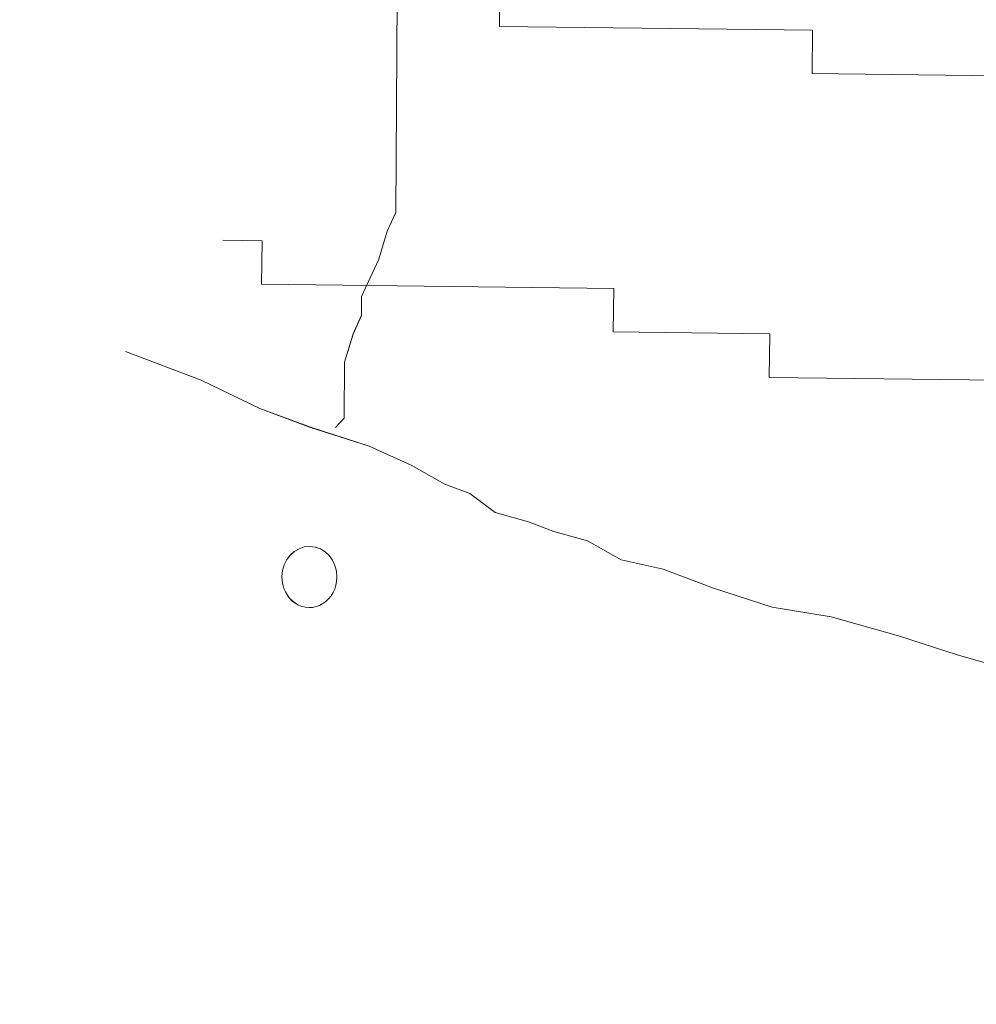
# Model space of a CAD drawing. Units: inches. Extents: x -466983 to 1020, y 324 to 318697.
# Tile 54 of 97: x 631.804 to 634.844, y 939.565 to 942.694. Entities that reach past the tile are written whole.
import ezdxf

# ---------------------------------------------------------------- set-up
doc = ezdxf.new("R2010")
doc.units = ezdxf.units.IN
doc.header["$MEASUREMENT"] = 0
doc.layers.add('A-FLOR-PATT', color=252, linetype='Continuous', lineweight=13)
doc.layers.add('A-FURN', color=8, linetype='Continuous', lineweight=18)

# ---------------------------------------------------------------- blocks, each defined once
blk = doc.blocks.new('L Shaped Sofa')
at = {"ltscale": 2}
for p, q in [((2434.5891, 747.5867), (2435.1737, 747.4213)), ((2435.1737, 747.4213), (2435.5146, 747.3113)), ((2435.5146, 747.3113), (2435.9043, 747.201)), ((2435.9043, 747.201), (2436.2455, 747.1452)), ((2436.2455, 747.1452), (2436.5864, 747.0351)), ((2436.5864, 747.0351), (2436.8785, 746.9253)), ((2436.8785, 746.9253), (2437.1222, 746.87)), ((2437.1222, 746.87), (2437.3167, 746.7606)), ((2437.3167, 746.7606), (2437.5115, 746.7055)), ((2437.5115, 746.7055), (2437.6576, 746.6506)), ((2437.6576, 746.6506), (2437.8524, 746.5955)), ((2437.8524, 746.5955), (2437.9981, 746.4863)), ((2437.9981, 746.4863), (2438.1442, 746.4314)), ((2438.1442, 746.4314), (2438.3387, 746.3221)), ((2438.3387, 746.3221), (2438.582, 746.2125)), ((2438.582, 746.2125), (2438.9229, 746.1025)), ((2438.7274, 746.0492), (2438.7765, 746.1032)), ((2438.9229, 746.1025), (2439.215, 745.9927)), ((2438.7254, 745.7239), (2438.7274, 746.0492)), ((2439.215, 745.9927), (2439.5556, 745.8284)), ((2434.2218, 745.8377), (2436.2633, 745.8128)), ((2436.2633, 745.8128), (2436.2603, 745.5609)), ((2439.5556, 745.8284), (2439.9938, 745.6637)), ((2438.6756, 745.5615), (2438.7254, 745.7239)), ((2436.2603, 745.5609), (2437.1676, 745.5498)), ((2438.6262, 745.4533), (2438.6756, 745.5615)), ((2437.1676, 745.5498), (2437.1645, 745.2979)), ((2438.6255, 745.3448), (2438.6262, 745.4533)), ((2438.5266, 745.1284), (2438.6255, 745.3448)), ((2437.1645, 745.2979), (2439.2061, 745.2729)), ((2439.2061, 745.2729), (2439.203, 745.021)), ((2438.4768, 744.966), (2438.5266, 745.1284)), ((2439.4298, 745.0182), (2439.203, 745.021)), ((2439.203, 745.021), (2439.4298, 745.0182)), ((2438.4273, 744.8578), (2438.4768, 744.966)), ((2438.4141, 742.6892), (2438.4273, 744.8578)), ((2433.5198, 744.0827), (2436.015, 744.0522)), ((2436.015, 744.0522), (2436.0119, 743.8003)), ((2436.0119, 743.8003), (2437.8266, 743.7781)), ((2437.8266, 743.7781), (2437.8235, 743.5262))]:
    blk.add_line(p, q, dxfattribs=at)
at = {"ltscale": 2, "extrusion": (0, 0, -1)}
for start_param, end_param in [(1.570796, 4.712389), (-1.570796, 1.570796)]:
    blk.add_ellipse((2438.9282, 746.9699), major_axis=(-0.0022, -0.1772), ratio=0.9, start_param=start_param, end_param=end_param, dxfattribs=at)

msp = doc.modelspace()

# ---------------------------------------------------------------- hatches: boundary and pattern name
at = {"layer": 'A-FLOR-PATT', "transparency": 33554572}
h = msp.add_hatch(dxfattribs=at)
h.set_pattern_fill('ANSI37', color=256, scale=30)
h.set_pattern_definition([(45, (-1212.4137, -290.035), (-2.6516504, 2.6516504), []), (135, (-1212.4137, -290.035), (-2.6516504, -2.6516504), [])])
h.paths.add_polyline_path([(901.8057, 1075.9377), (900.6144, 1075.9377), (900.6144, 1065.3856), (899.391, 1065.3856), (898.0911, 1065.3856), (892.8356, 1058.7098, -0.258377), (892.1875, 1058.3509), (879.9848, 1058.3509, -0.20177), (879.4382, 1058.5808), (874.0812, 1065.3856), (872.7813, 1065.3856), (871.5579, 1065.3856), (871.5579, 1075.9377), (813.8057, 1075.9377), (813.8057, 1044.7922), (832.3947, 1044.7922, -0.394795), (848.6602, 1028.5356), (848.6602, 1009.9377), (901.8057, 1009.9377), (901.8057, 1015.9377), (901.3057, 1015.9377), (871.3057, 1015.9377), (871.3057, 1017.2502), (871.3344, 1017.2502, -0.401453), (901.3057, 1045.9377), (901.8057, 1045.9377)])
edge = h.paths.add_edge_path(flags=16)
edge.add_line((847.7731, 1068.9486), (847.7731, 1073.7088))
edge.add_arc((849.2269, 1073.7088), 1.4538, 90, 180, ccw=False)
edge.add_line((849.2269, 1075.1627), (864.4921, 1075.1627))
edge.add_arc((864.4921, 1073.7088), 1.4538, 0, 90, ccw=False)
edge.add_line((865.9459, 1073.7088), (865.9459, 1069.0035))
edge.add_arc((832.6447, 1068.9761), 33.3012, -20.61234, 0.04725, ccw=False)
edge.add_ellipse((856.8595, 1058.48), major_axis=(0, 10.2131), ratio=0.6859192, start_angle=100.00884, end_angle=259.99116, ccw=False)
edge.add_arc((881.0742, 1068.9761), 33.3012, 180.04725, 200.61234, ccw=False)
h.paths.add_polyline_path([(853.1456, 1066.4815), (853.1456, 1066.4534), (853.1463, 1066.4534, 0.433107), (852.9166, 1066.6849), (852.9166, 1066.4534), (853.1456, 1066.4534), (853.1456, 1066.4815), (853.088, 1066.6122, 0.697939), (852.6995, 1066.4534), (852.7003, 1066.4534), (852.7003, 1066.4815), (852.9166, 1067.0012), (852.9166, 1066.6849, -0.396254)], flags=0)
h.paths.add_polyline_path([(861.0187, 1066.4815), (861.0187, 1066.4534), (861.0194, 1066.4534, 0.416404), (860.8024, 1066.6849), (860.8024, 1066.4534), (861.0187, 1066.4534), (861.0187, 1066.4815), (860.9672, 1066.6053, 0.713344), (860.5726, 1066.4534), (860.5734, 1066.4534), (860.5734, 1066.4815), (860.8024, 1067.0012), (860.8024, 1066.6849, -0.379973)], flags=0)
edge = h.paths.add_edge_path(flags=0)
edge.add_spline(control_points=[(861.1298, 1065.7855), (861.4661, 1065.2478), (861.6134, 1065.0161), (861.9833, 1064.3736), (862.1924, 1063.9443), (862.5614, 1063.0391), (862.7212, 1062.5633), (862.9865, 1061.5781), (863.092, 1061.0689), (863.2452, 1060.031), (863.293, 1059.5025), (863.3295, 1058.4409), (863.3181, 1057.9078), (863.2366, 1056.8518), (863.1664, 1056.3289), (862.9695, 1055.308), (862.8427, 1054.8099), (862.5365, 1053.8522), (862.3571, 1053.3927), (861.9514, 1052.5249), (861.7251, 1052.1166), (861.233, 1051.3622), (860.9672, 1051.0162), (860.4048, 1050.3949), (860.1082, 1050.1197), (859.4937, 1049.6461), (859.1758, 1049.4476), (858.5276, 1049.1299), (858.1973, 1049.0107), (857.5315, 1048.8518), (857.1959, 1048.8121), (856.5249, 1048.812), (856.1894, 1048.8515), (855.5236, 1049.0101), (855.1933, 1049.1291), (854.545, 1049.4465), (854.2271, 1049.6449), (853.6124, 1050.1183), (853.3158, 1050.3933), (852.7533, 1051.0143), (852.4874, 1051.3602), (851.9952, 1052.1144), (851.7688, 1052.5225), (851.3629, 1053.3902), (851.1834, 1053.8496), (850.877, 1054.8071), (850.7501, 1055.3051), (850.553, 1056.326), (850.4827, 1056.8488), (850.401, 1057.9048), (850.3895, 1058.4379), (850.4257, 1059.4995), (850.4734, 1060.0281), (850.6265, 1061.066), (850.7318, 1061.5753), (850.9969, 1062.5605), (851.1567, 1063.0365), (851.5254, 1063.9418), (851.7345, 1064.3712), (852.1056, 1065.0164), (852.2544, 1065.2503), (852.6082, 1065.7335)], knot_values=[3.915332, 3.915332, 3.915332, 3.915332, 4.013468, 4.013468, 4.175532, 4.175532, 4.337596, 4.337596, 4.49966, 4.49966, 4.661724, 4.661724, 4.823788, 4.823788, 4.985852, 4.985852, 5.147916, 5.147916, 5.30998, 5.30998, 5.472044, 5.472044, 5.634109, 5.634109, 5.796173, 5.796173, 5.958237, 5.958237, 6.120301, 6.120301, 6.282365, 6.282365, 6.444429, 6.444429, 6.606493, 6.606493, 6.768557, 6.768557, 6.930621, 6.930621, 7.092685, 7.092685, 7.254749, 7.254749, 7.416813, 7.416813, 7.578878, 7.578878, 7.740942, 7.740942, 7.903006, 7.903006, 8.06507, 8.06507, 8.227134, 8.227134, 8.389198, 8.389198, 8.551262, 8.551262, 8.65037, 8.65037, 8.65037, 8.65037], degree=3, periodic=0)
edge.add_line((852.6421, 1065.7855), (861.1298, 1065.7855))
edge = h.paths.add_edge_path(flags=0)
edge.add_ellipse((856.8496, 1057.7432), major_axis=(0, 7.7921), ratio=0.687861, start_angle=0, end_angle=360)
h.paths.add_polyline_path([(848.8634, 1069.3891), (848.8634, 1073.9605, -0.414214), (849.9538, 1075.0508), (863.7652, 1075.0508, -0.414214), (864.8555, 1073.9605), (864.8555, 1069.3891, -0.388936), (864.5237, 1069.027, -0.043561), (849.1953, 1069.027, -0.388936)], flags=0)
h.paths.add_polyline_path([(853.1006, 1068.1122, -1), (852.6775, 1068.1122, -1)], flags=0)
edge = h.paths.add_edge_path(flags=0)
edge.add_ellipse((856.8595, 1057.3378), major_axis=(0, 2.207), ratio=0.657164, start_angle=0, end_angle=360)
h.paths.add_polyline_path([(861.0415, 1068.1122, -1), (860.6184, 1068.1122, -1)], flags=0)
edge = h.paths.add_edge_path()
edge.add_line((573.9537, 1057.3412), (573.9537, 1075.9377))
edge.add_line((573.9537, 1075.9377), (558.7308, 1075.9377))
edge.add_line((558.7308, 1075.9377), (558.7308, 1065.3856))
edge.add_line((558.7308, 1065.3856), (557.5074, 1065.3856))
edge.add_line((557.5074, 1065.3856), (556.2075, 1065.3856))
edge.add_line((556.2075, 1065.3856), (550.952, 1058.7098))
edge.add_arc((550.3039, 1059.1155), 0.7646, 270, 327.9483, ccw=False)
edge.add_line((550.3039, 1058.3509), (538.1012, 1058.3509))
edge.add_arc((538.1012, 1059.1155), 0.7646, 224.3704, 270, ccw=False)
edge.add_line((537.5546, 1058.5808), (532.1976, 1065.3856))
edge.add_line((532.1976, 1065.3856), (530.8977, 1065.3856))
edge.add_line((530.8977, 1065.3856), (529.6743, 1065.3856))
edge.add_line((529.6743, 1065.3856), (529.6743, 1075.9377))
edge.add_line((529.6743, 1075.9377), (520.8057, 1075.9377))
edge.add_line((520.8057, 1075.9377), (520.8057, 1045.9377))
edge.add_line((520.8057, 1045.9377), (521.3057, 1045.9377))
edge.add_arc((521.3057, 1015.9377), 30, 2.50749, 90, ccw=False)
edge.add_line((551.277, 1017.2502), (551.3057, 1017.2502))
edge.add_line((551.3057, 1017.2502), (551.3057, 1015.9377))
edge.add_line((551.3057, 1015.9377), (520.8057, 1015.9377))
edge.add_line((520.8057, 1015.9377), (520.8057, 1009.9377))
edge.add_line((520.8057, 1009.9377), (559.1913, 1010.4022))
edge.add_arc((559.1913, 1011.856), 1.4538, 180, 270, ccw=False)
edge.add_line((557.7375, 1011.856), (557.7375, 1016.5613))
edge.add_arc((591.0386, 1016.5888), 33.3012, 159.38766, 180.04725, ccw=False)
edge.add_ellipse((566.8239, 1027.0848), major_axis=(0, 10.2131), ratio=0.6859192, start_angle=280.00884, end_angle=439.99116, ccw=False)
edge.add_arc((542.6091, 1016.5888), 33.3012, 0.04725, 20.61234, ccw=False)
edge.add_line((575.9103, 1016.6162), (575.9103, 1011.856))
edge.add_arc((574.4565, 1011.856), 1.4538, -90, 0, ccw=False)
edge.add_line((574.4565, 1010.4022), (608.8057, 1009.9377))
edge.add_line((608.8057, 1009.9377), (608.8057, 1041.0857))
edge.add_line((608.8057, 1041.0857), (590.2179, 1041.0857))
edge.add_arc((590.775, 1057.9074), 16.8309, 181.92775, 268.10321, ccw=False)
edge = h.paths.add_edge_path()
edge.add_ellipse((494.2443, 583.6204), major_axis=(0, 10.2131), ratio=0.6859192, start_angle=280.00884, end_angle=439.99116, ccw=False)
edge.add_arc((470.0296, 573.1243), 33.3012, 0.04725, 20.61234, ccw=False)
edge.add_line((503.3307, 573.1518), (503.3307, 568.3916))
edge.add_arc((501.8769, 568.3916), 1.4538, -90, 0, ccw=False)
edge.add_line((501.8769, 566.9377), (539.8057, 566.9377))
edge.add_line((539.8057, 566.9377), (539.8057, 572.9377))
edge.add_line((539.8057, 572.9377), (539.3057, 572.9377))
edge.add_line((539.3057, 572.9377), (509.3057, 572.9377))
edge.add_line((509.3057, 572.9377), (509.3057, 574.2502))
edge.add_line((509.3057, 574.2502), (509.3344, 574.2502))
edge.add_arc((539.3057, 572.9377), 30, 90, 177.49251, ccw=False)
edge.add_line((539.3057, 602.9377), (539.8057, 602.9377))
edge.add_line((539.8057, 602.9377), (539.8057, 626.9377))
edge.add_line((539.8057, 626.9377), (531.7718, 626.9377))
edge.add_line((531.7718, 626.9377), (531.7718, 616.3856))
edge.add_line((531.7718, 616.3856), (530.5484, 616.3856))
edge.add_line((530.5484, 616.3856), (529.2485, 616.3856))
edge.add_line((529.2485, 616.3856), (523.7105, 609.3509))
edge.add_line((523.7105, 609.3509), (510.7766, 609.3509))
edge.add_line((510.7766, 609.3509), (505.2386, 616.3856))
edge.add_line((505.2386, 616.3856), (503.9387, 616.3856))
edge.add_line((503.9387, 616.3856), (502.7153, 616.3856))
edge.add_line((502.7153, 616.3856), (502.7153, 626.9377))
edge.add_line((502.7153, 626.9377), (481.6983, 626.9377))
edge.add_line((481.6983, 626.9377), (481.6983, 610.995))
edge.add_arc((467.2703, 611.4728), 14.4359, 271.92775, 358.10321, ccw=False)
edge.add_line((467.7559, 597.0451), (451.8057, 597.0451))
edge.add_line((451.8057, 597.0451), (451.8057, 584.4035))
edge.add_line((451.8057, 584.4035), (451.8057, 566.9377))
edge.add_line((451.8057, 566.9377), (486.6117, 566.9377))
edge.add_arc((486.6117, 568.3916), 1.4538, 180, 270, ccw=False)
edge.add_line((485.1579, 568.3916), (485.1579, 573.0969))
edge.add_arc((518.4591, 573.1243), 33.3012, 159.38766, 180.04725, ccw=False)
h.paths.add_polyline_path([(836.2609, 1020.7328), (879.8898, 1020.7328), (879.8898, 1039.3902), (836.2609, 1039.3902)], flags=25)
h.paths.add_polyline_path([(549.9851, 1036.7492), (593.614, 1036.7492), (593.614, 1055.4065), (549.9851, 1055.4065)], flags=24)
h.paths.add_polyline_path([(475.123, 595.5959), (518.752, 595.5959), (518.752, 614.2532), (475.123, 614.2532)], flags=24)
h = msp.add_hatch(dxfattribs=at)
h.set_pattern_fill('ANSI37', color=256, scale=20)
h.set_pattern_definition([(45, (-1212.4137, -290.035), (-1.767767, 1.767767), []), (135, (-1212.4137, -290.035), (-1.767767, -1.767767), [])])
h.paths.add_polyline_path([(809.8057, 870.9377), (809.8057, 888.1519), (806.9985, 888.1519), (802.6624, 888.1519), (789.3832, 888.1519), (786.2846, 888.1519, -0.414214), (785.4991, 888.9374), (785.4991, 900.1959), (785.4991, 908.4696, -0.414214), (786.8082, 909.7787, -0.414214), (785.4991, 911.0878), (785.4991, 929.1015, -0.414214), (786.8082, 930.4106, -0.414214), (785.4991, 931.7197), (785.4991, 931.9039, -0.414214), (784.19, 930.5948), (766.7223, 930.5948, -0.412359), (765.4132, 931.8956, -0.413741), (764.1145, 930.5782), (744.5781, 930.422, -0.416556), (743.7864, 931.2075), (743.7864, 933.5153), (742.2154, 933.5153), (742.2154, 952.024, -0.001344), (743.7864, 952.1998), (743.7864, 953.9377), (678.5915, 953.9377), (678.5915, 951.1305), (678.5915, 946.7945), (678.5915, 933.5153), (678.5915, 930.4166, -0.414214), (677.806, 929.6312), (666.5475, 929.6312), (658.2738, 929.6312, -0.414214), (656.9647, 930.9403, -0.414214), (655.6556, 929.6312), (637.6419, 929.6312, -0.414214), (636.3328, 930.9403, -0.414214), (635.0237, 929.6312), (634.8395, 929.6312, -0.414214), (636.1486, 928.322), (636.1486, 910.8544, -0.412359), (634.8478, 909.5452, -0.413741), (636.1653, 908.2466), (636.3214, 888.7102, -0.416556), (635.5359, 887.9184), (633.2281, 887.9184), (633.2281, 886.3475), (614.7194, 886.3475, -0.001344), (614.5436, 887.9184), (612.8057, 887.9184), (612.8057, 834.9377), (612.8057, 752.9377), (612.8057, 748.9377), (612.8057, 697.9377), (654.8057, 697.9377), (654.8057, 701.9377), (715.8057, 701.9377), (715.8057, 737.4353), (774.2918, 737.4353), (774.2918, 795.9377), (809.8057, 795.9377)])
h.paths.add_polyline_path([(679.2761, 849.5757, 0.102523), (682.1475, 849.2608, -0.080461), (694.5428, 849.7725, -0.283899), (694.4822, 849.0082, 0.136605), (694.4068, 848.8103, -0.030441), (694.5428, 846.8929), (694.5428, 842.6198), (694.5428, 838.3466, -0.028219), (694.4246, 836.5684), (694.425, 836.5684, 0.196187), (694.4456, 836.2708, -0.302897), (694.5428, 835.467, -0.080461), (682.1475, 835.9787, 0.102523), (679.2761, 835.6638, -0.58611), (678.6457, 836.0169), (678.6457, 849.2227, -0.58611)], flags=16)
h.paths.add_polyline_path([(679.5173, 848.6515, 0.699597), (679.476, 848.6342, 1.20716), (679.1935, 848.7422, 0.010621)], flags=0)
h.paths.add_polyline_path([(679.4923, 836.5608, -0.013798), (679.9178, 836.6594, -0.071703), (682.8533, 837.1434, -0.165743), (682.1665, 839.1006), (682.1665, 842.6094), (682.1665, 846.0603, -0.240616), (683.4733, 848.6767, -0.068263), (693.9295, 849.0082), (693.7875, 848.7083), (693.7875, 849.0228, 0.067332), (683.4733, 848.6767, 0.240616), (682.1665, 846.0603), (682.1665, 842.6094), (682.1665, 839.1006, 0.23459), (683.461, 836.5513, 0.068093), (693.7875, 836.1955), (693.7875, 836.5104), (693.9296, 836.2102, -0.077215), (682.2421, 836.7815, 0.086627), (679.5283, 836.5701, -0.628402), (679.5029, 836.5735), (679.5029, 836.6071, 0.910458)], flags=0)
h.paths.add_polyline_path([(679.476, 848.6364), (679.2069, 848.647), (679.2069, 836.5718, 0.913566), (679.3645, 836.5861), (679.476, 836.5824)], flags=0)
h.paths.add_polyline_path([(679.2761, 829.8604, 0.102523), (682.1475, 829.5455, -0.080461), (694.5428, 830.0572, -0.283899), (694.4822, 829.2929, 0.136605), (694.4068, 829.095, -0.030441), (694.5428, 827.1776), (694.5428, 822.9045), (694.5428, 818.6314, -0.028219), (694.4246, 816.8531), (694.425, 816.8532, 0.196187), (694.4456, 816.5555, -0.302897), (694.5428, 815.7517, -0.080461), (682.1475, 816.2635, 0.102523), (679.2761, 815.9485, -0.58611), (678.6457, 816.3016), (678.6457, 829.5074, -0.58611)], flags=16)
h.paths.add_polyline_path([(679.5173, 828.9362, 0.699597), (679.476, 828.9189, 1.20716), (679.1935, 829.0269, 0.010621)], flags=0)
h.paths.add_polyline_path([(679.4923, 816.8456, -0.013798), (679.9178, 816.9441, -0.071703), (682.8533, 817.4281, -0.165743), (682.1665, 819.3853), (682.1665, 822.8941), (682.1665, 826.345, -0.240616), (683.4733, 828.9614, -0.068263), (693.9295, 829.2929), (693.7875, 828.9931), (693.7875, 829.3076, 0.067332), (683.4733, 828.9614, 0.240616), (682.1665, 826.345), (682.1665, 822.8941), (682.1665, 819.3853, 0.23459), (683.461, 816.836, 0.068093), (693.7875, 816.4802), (693.7875, 816.7952), (693.9296, 816.4949, -0.077215), (682.2421, 817.0662, 0.086627), (679.5283, 816.8549, -0.628402), (679.5029, 816.8582), (679.5029, 816.8918, 0.910458)], flags=0)
h.paths.add_polyline_path([(679.476, 828.9211), (679.2069, 828.9317), (679.2069, 816.8565, 0.913566), (679.3645, 816.8708), (679.476, 816.8671)], flags=0)
h.paths.add_polyline_path([(679.2761, 810.1451, 0.102523), (682.1475, 809.8302, -0.080461), (694.5428, 810.342, -0.3023), (694.4466, 809.5394, 0.10023), (694.4058, 809.3878, -0.03057), (694.5428, 807.4623), (694.5428, 803.1892), (694.5428, 798.9161, -0.03057), (694.4058, 796.9906, 0.10023), (694.4466, 796.839, -0.3023), (694.5428, 796.0365, -0.080461), (682.1475, 796.5482, 0.102523), (679.2761, 796.2333, -0.58611), (678.6457, 796.5863), (678.6457, 809.7921, -0.58611)], flags=16)
h.paths.add_polyline_path([(679.5173, 809.2417, 0.699597), (679.476, 809.2244, 1.20716), (679.1935, 809.3324, 0.010621)], flags=0)
h.paths.add_polyline_path([(679.4923, 797.151, -0.013798), (679.9178, 797.2496, -0.071703), (682.8533, 797.7336, -0.165743), (682.1665, 799.6908), (682.1665, 803.1996), (682.1665, 806.6505, -0.239349), (683.461, 809.2577, -0.072465), (694.4468, 809.5405, 0.197932), (694.425, 809.2405), (693.7875, 809.2985), (693.7875, 809.6135, 0.068093), (683.461, 809.2577, 0.239349), (682.1665, 806.6505), (682.1665, 803.1996), (682.1665, 799.6908, 0.235854), (683.4733, 797.1323, 0.067332), (693.7875, 796.7861), (693.7875, 797.1006), (694.425, 797.1586, 0.197932), (694.4468, 796.8586, -0.080419), (682.1557, 797.3795, 0.083867), (679.5283, 797.1603, -0.628402), (679.5029, 797.1637), (679.5029, 797.1973, 0.910458)], flags=0)
h.paths.add_polyline_path([(679.2069, 809.2372), (679.2069, 797.162, 0.913566), (679.3645, 797.1763), (679.476, 797.1726), (679.476, 809.2266)], flags=0)
h.paths.add_polyline_path([(695.3643, 853.2989), (728.2231, 853.2989), (728.2231, 771.1519), (695.3643, 771.1519)], flags=16)
h.paths.add_polyline_path([(696.0215, 852.6417), (727.5659, 852.6417), (727.5659, 771.809), (696.0215, 771.809)], flags=0)
h.paths.add_polyline_path([(679.2761, 788.7869, 0.102523), (682.1475, 788.472, -0.080461), (694.5428, 788.9837, -0.3023), (694.4466, 788.1812, 0.10023), (694.4058, 788.0296, -0.03057), (694.5428, 786.1041), (694.5428, 781.831), (694.5428, 777.5578, -0.03057), (694.4058, 775.6323, 0.10023), (694.4466, 775.4808, -0.3023), (694.5428, 774.6782, -0.080461), (682.1475, 775.19, 0.102523), (679.2761, 774.875, -0.58611), (678.6457, 775.2281), (678.6457, 788.4339, -0.58611)], flags=16)
h.paths.add_polyline_path([(679.5173, 787.8834, 0.699597), (679.476, 787.8662, 1.20716), (679.1935, 787.9742, 0.010621)], flags=0)
h.paths.add_polyline_path([(679.4923, 775.7928, -0.013798), (679.9178, 775.8914, -0.071703), (682.8533, 776.3753, -0.165743), (682.1665, 778.3325), (682.1665, 781.8414), (682.1665, 785.2922, -0.239349), (683.461, 787.8995, -0.072465), (694.4468, 788.1823, 0.197932), (694.425, 787.8823), (693.7875, 787.9403), (693.7875, 788.2553, 0.068093), (683.461, 787.8995, 0.239349), (682.1665, 785.2922), (682.1665, 781.8414), (682.1665, 778.3325, 0.235854), (683.4733, 775.7741, 0.067332), (693.7875, 775.4279), (693.7875, 775.7424), (694.425, 775.8004, 0.197932), (694.4468, 775.5004, -0.080419), (682.1557, 776.0212, 0.083867), (679.5283, 775.8021, -0.628402), (679.5029, 775.8054), (679.5029, 775.8391, 0.910458)], flags=0)
h.paths.add_polyline_path([(679.2069, 787.8789), (679.2069, 775.8038, 0.913566), (679.3645, 775.818), (679.476, 775.8144), (679.476, 787.8684)], flags=0)
h.paths.add_polyline_path([(704.641, 854.1204, -0.080461), (705.1527, 866.5157, 0.102523), (704.8378, 869.3871, -0.58611), (705.1908, 870.0174), (718.3966, 870.0174, -0.58611), (718.7496, 869.3871, 0.102523), (718.4347, 866.5157, -0.080461), (718.9465, 854.1204, -0.3023), (718.1439, 854.2166, 0.10023), (717.9924, 854.2574, -0.03057), (716.0668, 854.1204), (711.7937, 854.1204), (707.5206, 854.1204, -0.03057), (705.5951, 854.2574, 0.10023), (705.4435, 854.2166, -0.3023)], flags=16)
h.paths.add_polyline_path([(717.8462, 869.1459, 0.699597), (717.8289, 869.1872, 1.20716), (717.9369, 869.4697, 0.010621)], flags=0)
h.paths.add_polyline_path([(705.4631, 854.2164, -0.080419), (705.984, 866.5074, 0.083867), (705.7648, 869.1349, -0.628402), (705.7682, 869.1603), (705.8018, 869.1603, 0.910458), (705.7555, 869.1709, -0.013798), (705.8541, 868.7454, -0.071703), (706.3381, 865.8099, -0.165743), (708.2953, 866.4967), (711.8041, 866.4967), (715.255, 866.4967, -0.239349), (717.8622, 865.2022, -0.072465), (718.145, 854.2164, 0.197932), (717.845, 854.2382), (717.903, 854.8757), (718.218, 854.8757, 0.068093), (717.8622, 865.2022, 0.239349), (715.255, 866.4967), (711.8041, 866.4967), (708.2953, 866.4967, 0.235854), (705.7368, 865.1898, 0.067332), (705.3906, 854.8757), (705.7051, 854.8757), (705.7631, 854.2382, 0.197932)], flags=16)
h.paths.add_polyline_path([(705.7665, 869.4563, 0.913566), (705.7808, 869.2987), (705.7771, 869.1872), (717.8311, 869.1872), (717.8417, 869.4563)], flags=0)
h.paths.add_polyline_path([(729.0446, 842.6198), (729.0446, 846.8929, -0.03057), (729.1817, 848.8184, 0.10023), (729.1408, 848.9699, -0.3023), (729.0446, 849.7725, -0.080461), (741.4399, 849.2608, 0.102523), (744.3113, 849.5757, -0.58611), (744.9417, 849.2227), (744.9417, 836.0169, -0.58611), (744.3113, 835.6638, 0.102523), (741.4399, 835.9787, -0.080461), (729.0446, 835.467, -0.3023), (729.1408, 836.2696, 0.10023), (729.1817, 836.4211, -0.03057), (729.0446, 838.3466)], flags=16)
h.paths.add_polyline_path([(744.1115, 836.5846, 1.20716), (744.3939, 836.4766, 0.010621), (744.0701, 836.5673, 0.699597)], flags=0)
h.paths.add_polyline_path([(729.1407, 836.2684, 0.197932), (729.1624, 836.5684), (729.7999, 836.5104), (729.7999, 836.1955, 0.068093), (740.1264, 836.5513, 0.239349), (741.4209, 839.1585), (741.4209, 842.6094), (741.4209, 846.1182, 0.235854), (740.1141, 848.6767, 0.067332), (729.7999, 849.0228), (729.7999, 848.7083), (729.1624, 848.6503, 0.197932), (729.1407, 848.9504, -0.080419), (741.4317, 848.4295, 0.083867), (744.0591, 848.6486, -0.628402), (744.0845, 848.6453), (744.0845, 848.6117, 0.910458), (744.0951, 848.6579, -0.013798), (743.6696, 848.5594, -0.071703), (740.7341, 848.0754, -0.165743), (741.4209, 846.1182), (741.4209, 842.6094), (741.4209, 839.1585, -0.239349), (740.1264, 836.5513, -0.072465)], flags=0)
h.paths.add_polyline_path([(729.0446, 830.0572, -0.080461), (741.4399, 829.5455, 0.102523), (744.3113, 829.8604, -0.58611), (744.9417, 829.5074), (744.9417, 816.3016, -0.58611), (744.3113, 815.9485, 0.102523), (741.4399, 816.2635, -0.080461), (729.0446, 815.7517, -0.3023), (729.1408, 816.5543, 0.10023), (729.1817, 816.7058, -0.03057), (729.0446, 818.6314), (729.0446, 822.9045), (729.0446, 827.1776, -0.03057), (729.1817, 829.1031, 0.10023), (729.1408, 829.2547, -0.3023)], flags=16)
h.paths.add_polyline_path([(744.1115, 816.8693, 1.20716), (744.3939, 816.7613, 0.010621), (744.0701, 816.852, 0.699597)], flags=0)
h.paths.add_polyline_path([(729.1407, 829.2351, -0.080419), (741.4317, 828.7142, 0.083867), (744.0591, 828.9334, -0.628402), (744.0845, 828.93), (744.0845, 828.8964, 0.910458), (744.0951, 828.9427, -0.013798), (743.6696, 828.8441, -0.071703), (740.7341, 828.3601, -0.165743), (741.4209, 826.4029), (741.4209, 822.8941), (741.4209, 819.4432, -0.239349), (740.1264, 816.836, -0.072465), (729.1407, 816.5531, 0.197932), (729.1624, 816.8532), (729.7999, 816.7952), (729.7999, 816.4802, 0.068093), (740.1264, 816.836, 0.239349), (741.4209, 819.4432), (741.4209, 822.8941), (741.4209, 826.4029, 0.235854), (740.1141, 828.9614, 0.067332), (729.7999, 829.3076), (729.7999, 828.9931), (729.1624, 828.9351, 0.197932)], flags=16)
h.paths.add_polyline_path([(729.0446, 810.342, -0.080461), (741.4399, 809.8302, 0.102523), (744.3113, 810.1451, -0.58611), (744.9417, 809.7921), (744.9417, 796.5863, -0.58611), (744.3113, 796.2333, 0.102523), (741.4399, 796.5482, -0.080461), (729.0446, 796.0365, -0.283899), (729.1052, 796.8007, 0.136605), (729.1806, 796.9987, -0.030441), (729.0446, 798.9161), (729.0446, 803.1892), (729.0446, 807.4623, -0.028219), (729.1628, 809.2406), (729.1624, 809.2405, 0.196187), (729.1418, 809.5382, -0.302897)], flags=16)
h.paths.add_polyline_path([(744.1115, 797.1748, 1.20716), (744.3939, 797.0668, 0.010621), (744.0701, 797.1575, 0.699597)], flags=0)
h.paths.add_polyline_path([(741.3453, 809.0275, 0.086627), (744.0591, 809.2388, -0.628402), (744.0845, 809.2355), (744.0845, 809.2019, 0.910458), (744.0951, 809.2481, -0.013798), (743.6696, 809.1496, -0.071703), (740.7341, 808.6656, -0.165743), (741.4209, 806.7084), (741.4209, 803.1996), (741.4209, 799.7487, -0.240616), (740.1141, 797.1323, -0.068263), (729.658, 796.8008), (729.7999, 797.1006), (729.7999, 796.7861, 0.067332), (740.1141, 797.1323, 0.240616), (741.4209, 799.7487), (741.4209, 803.1996), (741.4209, 806.7084, 0.23459), (740.1264, 809.2577, 0.068093), (729.7999, 809.6135), (729.7999, 809.2985), (729.6578, 809.5988, -0.077215)], flags=0)
h.paths.add_polyline_path([(704.641, 770.3304, -0.283899), (705.4053, 770.2697, 0.136605), (705.6032, 770.1944, -0.030441), (707.5206, 770.3304), (711.7937, 770.3304), (716.0668, 770.3304, -0.028219), (717.8451, 770.2122), (717.845, 770.2126, 0.196187), (718.1427, 770.2331, -0.302897), (718.9465, 770.3304, -0.080461), (718.4347, 757.9351, 0.102523), (718.7496, 755.0637, -0.58611), (718.3966, 754.4333), (705.1908, 754.4333, -0.58611), (704.8378, 755.0637, 0.102523), (705.1527, 757.9351, -0.080461)], flags=16)
h.paths.add_polyline_path([(705.762, 755.3048, 0.699597), (705.7793, 755.2635, 1.20716), (705.6713, 754.9811, 0.010621)], flags=0)
h.paths.add_polyline_path([(705.4053, 769.717), (705.7051, 769.5751), (705.3906, 769.5751, 0.067332), (705.7368, 759.2609, 0.240616), (708.3532, 757.954), (711.8041, 757.954), (715.3129, 757.954, 0.23459), (717.8622, 759.2485, 0.068093), (718.218, 769.5751), (717.903, 769.5751), (718.2033, 769.7172, -0.077215), (717.632, 758.0297, 0.086627), (717.8433, 755.3159, -0.628402), (717.84, 755.2904), (717.8064, 755.2904, 0.910458), (717.8526, 755.2799, -0.013798), (717.7541, 755.7053, -0.071703), (717.2701, 758.6409, -0.165743), (715.3129, 757.954), (711.8041, 757.954), (708.3532, 757.954, -0.240616), (705.7368, 759.2609, -0.068263)], flags=0)
h.paths.add_polyline_path([(729.0446, 788.9837, -0.080461), (741.4399, 788.472, 0.102523), (744.3113, 788.7869, -0.58611), (744.9417, 788.4339), (744.9417, 775.2281, -0.58611), (744.3113, 774.875, 0.102523), (741.4399, 775.19, -0.080461), (729.0446, 774.6782, -0.283899), (729.1052, 775.4425, 0.136605), (729.1806, 775.6405, -0.030441), (729.0446, 777.5578), (729.0446, 781.831), (729.0446, 786.1041, -0.028219), (729.1628, 787.8823), (729.1624, 787.8823, 0.196187), (729.1418, 788.1799, -0.302897)], flags=16)
h.paths.add_polyline_path([(744.1115, 775.8165, 1.20716), (744.3939, 775.7086, 0.010621), (744.0701, 775.7993, 0.699597)], flags=0)
h.paths.add_polyline_path([(741.3453, 787.6692, 0.086627), (744.0591, 787.8806, -0.628402), (744.0845, 787.8773), (744.0845, 787.8437, 0.910458), (744.0951, 787.8899, -0.013798), (743.6696, 787.7913, -0.071703), (740.7341, 787.3074, -0.165743), (741.4209, 785.3502), (741.4209, 781.8414), (741.4209, 778.3905, -0.240616), (740.1141, 775.7741, -0.068263), (729.658, 775.4425), (729.7999, 775.7424), (729.7999, 775.4279, 0.067332), (740.1141, 775.7741, 0.240616), (741.4209, 778.3905), (741.4209, 781.8414), (741.4209, 785.3502, 0.23459), (740.1264, 787.8995, 0.068093), (729.7999, 788.2553), (729.7999, 787.9403), (729.6578, 788.2405, -0.077215)], flags=0)
h.paths.add_polyline_path([(744.1115, 848.6364), (744.1115, 836.5824), (744.3805, 836.5718), (744.3805, 848.647, 0.913566), (744.2229, 848.6327)], flags=0)
h.paths.add_polyline_path([(744.2229, 828.9174), (744.1115, 828.9211), (744.1115, 816.8671), (744.3805, 816.8565), (744.3805, 828.9317, 0.913566)], flags=0)
h.paths.add_polyline_path([(717.8311, 755.2635), (705.7771, 755.2635), (705.7665, 754.9945), (717.8417, 754.9945, 0.913566), (717.8274, 755.1521)], flags=0)
h.paths.add_polyline_path([(744.2229, 809.2229), (744.1115, 809.2266), (744.1115, 797.1726), (744.3805, 797.162), (744.3805, 809.2372, 0.913566)], flags=0)
h.paths.add_polyline_path([(744.1115, 787.8684), (744.1115, 775.8144), (744.3805, 775.8038), (744.3805, 787.8789, 0.913566), (744.2229, 787.8647)], flags=0)
h.paths.add_polyline_path([(678.8774, 877.1228), (737.6127, 877.1228), (737.6127, 899.5116), (678.8774, 899.5116)], flags=24)

# ---------------------------------------------------------------- linework, layer by layer
at = {"layer": 'A-FURN', "ltscale": 2}
for p, q in [((633.0067, 943.2696), (632.9994, 942.0807)), ((633.0067, 943.2696), (632.9994, 942.0807)), ((633.0067, 943.2696), (632.9994, 942.0807)), ((633.0067, 943.2696), (632.9994, 942.0807)), ((633.0067, 943.2696), (632.9994, 942.0807)), ((633.0067, 943.2696), (632.9994, 942.0807)), ((633.3288, 942.6726), (633.3305, 942.8107)), ((633.3288, 942.6726), (633.3305, 942.8107)), ((633.3288, 942.6726), (633.3305, 942.8107)), ((633.3288, 942.6726), (633.3305, 942.8107)), ((633.3288, 942.6726), (633.3305, 942.8107)), ((633.3288, 942.6726), (633.3305, 942.8107)), ((634.3236, 942.6605), (633.3288, 942.6726)), ((634.3236, 942.6605), (633.3288, 942.6726)), ((634.3236, 942.6605), (633.3288, 942.6726)), ((634.3236, 942.6605), (633.3288, 942.6726)), ((634.3236, 942.6605), (633.3288, 942.6726)), ((634.3236, 942.6605), (633.3288, 942.6726)), ((634.3219, 942.5224), (634.3236, 942.6605)), ((634.3219, 942.5224), (634.3236, 942.6605)), ((634.3219, 942.5224), (634.3236, 942.6605)), ((634.3219, 942.5224), (634.3236, 942.6605)), ((634.3219, 942.5224), (634.3236, 942.6605)), ((634.3219, 942.5224), (634.3236, 942.6605)), ((635.6899, 942.5057), (634.3219, 942.5224)), ((635.6899, 942.5057), (634.3219, 942.5224)), ((635.6899, 942.5057), (634.3219, 942.5224)), ((635.6899, 942.5057), (634.3219, 942.5224)), ((635.6899, 942.5057), (634.3219, 942.5224)), ((635.6899, 942.5057), (634.3219, 942.5224)), ((632.9994, 942.0807), (632.9723, 942.0214)), ((632.9994, 942.0807), (632.9723, 942.0214)), ((632.9994, 942.0807), (632.9723, 942.0214)), ((632.9994, 942.0807), (632.9723, 942.0214)), ((632.9994, 942.0807), (632.9723, 942.0214)), ((632.9994, 942.0807), (632.9723, 942.0214)), ((632.9723, 942.0214), (632.945, 941.9324)), ((632.9723, 942.0214), (632.945, 941.9324)), ((632.9723, 942.0214), (632.945, 941.9324)), ((632.9723, 942.0214), (632.945, 941.9324)), ((632.9723, 942.0214), (632.945, 941.9324)), ((632.9723, 942.0214), (632.945, 941.9324)), ((632.4499, 941.9928), (632.5742, 941.9912)), ((632.5742, 941.9912), (632.4499, 941.9928)), ((632.4499, 941.9928), (632.5742, 941.9912)), ((632.5742, 941.9912), (632.4499, 941.9928)), ((632.4499, 941.9928), (632.5742, 941.9912)), ((632.5742, 941.9912), (632.4499, 941.9928)), ((632.4499, 941.9928), (632.5742, 941.9912)), ((632.5742, 941.9912), (632.4499, 941.9928)), ((632.4499, 941.9928), (632.5742, 941.9912)), ((632.5742, 941.9912), (632.4499, 941.9928)), ((632.4499, 941.9928), (632.5742, 941.9912)), ((632.5742, 941.9912), (632.4499, 941.9928)), ((632.5725, 941.8531), (632.5742, 941.9912)), ((632.5725, 941.8531), (632.5742, 941.9912)), ((632.5725, 941.8531), (632.5742, 941.9912)), ((632.5725, 941.8531), (632.5742, 941.9912)), ((632.5725, 941.8531), (632.5742, 941.9912)), ((632.5725, 941.8531), (632.5742, 941.9912)), ((632.945, 941.9324), (632.8908, 941.8137)), ((632.945, 941.9324), (632.8908, 941.8137)), ((632.945, 941.9324), (632.8908, 941.8137)), ((632.945, 941.9324), (632.8908, 941.8137)), ((632.945, 941.9324), (632.8908, 941.8137)), ((632.945, 941.9324), (632.8908, 941.8137)), ((633.6917, 941.8395), (632.5725, 941.8531)), ((633.6917, 941.8395), (632.5725, 941.8531)), ((633.6917, 941.8395), (632.5725, 941.8531)), ((633.6917, 941.8395), (632.5725, 941.8531)), ((633.6917, 941.8395), (632.5725, 941.8531)), ((633.6917, 941.8395), (632.5725, 941.8531)), ((633.69, 941.7014), (633.6917, 941.8395)), ((633.69, 941.7014), (633.6917, 941.8395)), ((633.69, 941.7014), (633.6917, 941.8395)), ((633.69, 941.7014), (633.6917, 941.8395)), ((633.69, 941.7014), (633.6917, 941.8395)), ((633.69, 941.7014), (633.6917, 941.8395)), ((632.8908, 941.8137), (632.8904, 941.7543)), ((632.8908, 941.8137), (632.8904, 941.7543)), ((632.8908, 941.8137), (632.8904, 941.7543)), ((632.8908, 941.8137), (632.8904, 941.7543)), ((632.8908, 941.8137), (632.8904, 941.7543)), ((632.8908, 941.8137), (632.8904, 941.7543)), ((632.8904, 941.7543), (632.8633, 941.695)), ((632.8904, 941.7543), (632.8633, 941.695)), ((632.8904, 941.7543), (632.8633, 941.695)), ((632.8904, 941.7543), (632.8633, 941.695)), ((632.8904, 941.7543), (632.8633, 941.695)), ((632.8904, 941.7543), (632.8633, 941.695)), ((634.1875, 941.6953), (633.69, 941.7014)), ((634.1875, 941.6953), (633.69, 941.7014)), ((634.1875, 941.6953), (633.69, 941.7014)), ((634.1875, 941.6953), (633.69, 941.7014)), ((634.1875, 941.6953), (633.69, 941.7014)), ((634.1875, 941.6953), (633.69, 941.7014)), ((634.1858, 941.5572), (634.1875, 941.6953)), ((634.1858, 941.5572), (634.1875, 941.6953)), ((634.1858, 941.5572), (634.1875, 941.6953)), ((634.1858, 941.5572), (634.1875, 941.6953)), ((634.1858, 941.5572), (634.1875, 941.6953)), ((634.1858, 941.5572), (634.1875, 941.6953)), ((632.8633, 941.695), (632.836, 941.6059)), ((632.8633, 941.695), (632.836, 941.6059)), ((632.8633, 941.695), (632.836, 941.6059)), ((632.8633, 941.695), (632.836, 941.6059)), ((632.8633, 941.695), (632.836, 941.6059)), ((632.8633, 941.695), (632.836, 941.6059)), ((632.3809, 941.5486), (632.1407, 941.6389)), ((632.3809, 941.5486), (632.1407, 941.6389)), ((632.3809, 941.5486), (632.1407, 941.6389)), ((632.3809, 941.5486), (632.1407, 941.6389)), ((632.3809, 941.5486), (632.1407, 941.6389)), ((632.3809, 941.5486), (632.1407, 941.6389)), ((632.836, 941.6059), (632.8349, 941.4276)), ((632.836, 941.6059), (632.8349, 941.4276)), ((632.836, 941.6059), (632.8349, 941.4276)), ((632.836, 941.6059), (632.8349, 941.4276)), ((632.836, 941.6059), (632.8349, 941.4276)), ((632.836, 941.6059), (632.8349, 941.4276)), ((632.5676, 941.4586), (632.3809, 941.5486)), ((632.5676, 941.4586), (632.3809, 941.5486)), ((632.5676, 941.4586), (632.3809, 941.5486)), ((632.5676, 941.4586), (632.3809, 941.5486)), ((632.5676, 941.4586), (632.3809, 941.5486)), ((632.5676, 941.4586), (632.3809, 941.5486)), ((635.305, 941.5435), (634.1858, 941.5572)), ((635.305, 941.5435), (634.1858, 941.5572)), ((635.305, 941.5435), (634.1858, 941.5572)), ((635.305, 941.5435), (634.1858, 941.5572)), ((635.305, 941.5435), (634.1858, 941.5572)), ((635.305, 941.5435), (634.1858, 941.5572)), ((632.7278, 941.3984), (632.5676, 941.4586)), ((632.7278, 941.3984), (632.5676, 941.4586)), ((632.7278, 941.3984), (632.5676, 941.4586)), ((632.7278, 941.3984), (632.5676, 941.4586)), ((632.7278, 941.3984), (632.5676, 941.4586)), ((632.7278, 941.3984), (632.5676, 941.4586)), ((632.8349, 941.4276), (632.808, 941.398)), ((632.8349, 941.4276), (632.808, 941.398)), ((632.8349, 941.4276), (632.808, 941.398)), ((632.8349, 941.4276), (632.808, 941.398)), ((632.8349, 941.4276), (632.808, 941.398)), ((632.8349, 941.4276), (632.808, 941.398)), ((632.9146, 941.338), (632.7278, 941.3984)), ((632.9146, 941.338), (632.7278, 941.3984)), ((632.9146, 941.338), (632.7278, 941.3984)), ((632.9146, 941.338), (632.7278, 941.3984)), ((632.9146, 941.338), (632.7278, 941.3984)), ((632.9146, 941.338), (632.7278, 941.3984)), ((633.048, 941.278), (632.9146, 941.338)), ((633.048, 941.278), (632.9146, 941.338)), ((633.048, 941.278), (632.9146, 941.338)), ((633.048, 941.278), (632.9146, 941.338)), ((633.048, 941.278), (632.9146, 941.338)), ((633.048, 941.278), (632.9146, 941.338)), ((633.1547, 941.218), (633.048, 941.278)), ((633.1547, 941.218), (633.048, 941.278)), ((633.1547, 941.218), (633.048, 941.278)), ((633.1547, 941.218), (633.048, 941.278)), ((633.1547, 941.218), (633.048, 941.278)), ((633.1547, 941.218), (633.048, 941.278)), ((633.2347, 941.1879), (633.1547, 941.218)), ((633.2347, 941.1879), (633.1547, 941.218)), ((633.2347, 941.1879), (633.1547, 941.218)), ((633.2347, 941.1879), (633.1547, 941.218)), ((633.2347, 941.1879), (633.1547, 941.218)), ((633.2347, 941.1879), (633.1547, 941.218)), ((633.3146, 941.1281), (633.2347, 941.1879)), ((633.3146, 941.1281), (633.2347, 941.1879)), ((633.3146, 941.1281), (633.2347, 941.1879)), ((633.3146, 941.1281), (633.2347, 941.1879)), ((633.3146, 941.1281), (633.2347, 941.1879)), ((633.3146, 941.1281), (633.2347, 941.1879)), ((633.4214, 941.0979), (633.3146, 941.1281)), ((633.4214, 941.0979), (633.3146, 941.1281)), ((633.4214, 941.0979), (633.3146, 941.1281)), ((633.4214, 941.0979), (633.3146, 941.1281)), ((633.4214, 941.0979), (633.3146, 941.1281)), ((633.4214, 941.0979), (633.3146, 941.1281)), ((633.5015, 941.0678), (633.4214, 941.0979)), ((633.5015, 941.0678), (633.4214, 941.0979)), ((633.5015, 941.0678), (633.4214, 941.0979)), ((633.5015, 941.0678), (633.4214, 941.0979)), ((633.5015, 941.0678), (633.4214, 941.0979)), ((633.5015, 941.0678), (633.4214, 941.0979)), ((633.6083, 941.0376), (633.5015, 941.0678)), ((633.6083, 941.0376), (633.5015, 941.0678)), ((633.6083, 941.0376), (633.5015, 941.0678)), ((633.6083, 941.0376), (633.5015, 941.0678)), ((633.6083, 941.0376), (633.5015, 941.0678)), ((633.6083, 941.0376), (633.5015, 941.0678)), ((633.715, 940.9776), (633.6083, 941.0376)), ((633.715, 940.9776), (633.6083, 941.0376)), ((633.715, 940.9776), (633.6083, 941.0376)), ((633.715, 940.9776), (633.6083, 941.0376)), ((633.715, 940.9776), (633.6083, 941.0376)), ((633.715, 940.9776), (633.6083, 941.0376)), ((633.8485, 940.9473), (633.715, 940.9776)), ((633.8485, 940.9473), (633.715, 940.9776)), ((633.8485, 940.9473), (633.715, 940.9776)), ((633.8485, 940.9473), (633.715, 940.9776)), ((633.8485, 940.9473), (633.715, 940.9776)), ((633.8485, 940.9473), (633.715, 940.9776)), ((634.0087, 940.8871), (633.8485, 940.9473)), ((634.0087, 940.8871), (633.8485, 940.9473)), ((634.0087, 940.8871), (633.8485, 940.9473)), ((634.0087, 940.8871), (633.8485, 940.9473)), ((634.0087, 940.8871), (633.8485, 940.9473)), ((634.0087, 940.8871), (633.8485, 940.9473)), ((634.1956, 940.8267), (634.0087, 940.8871)), ((634.1956, 940.8267), (634.0087, 940.8871)), ((634.1956, 940.8267), (634.0087, 940.8871)), ((634.1956, 940.8267), (634.0087, 940.8871)), ((634.1956, 940.8267), (634.0087, 940.8871)), ((634.1956, 940.8267), (634.0087, 940.8871)), ((634.3826, 940.7961), (634.1956, 940.8267)), ((634.3826, 940.7961), (634.1956, 940.8267)), ((634.3826, 940.7961), (634.1956, 940.8267)), ((634.3826, 940.7961), (634.1956, 940.8267)), ((634.3826, 940.7961), (634.1956, 940.8267)), ((634.3826, 940.7961), (634.1956, 940.8267)), ((634.5963, 940.7357), (634.3826, 940.7961)), ((634.5963, 940.7357), (634.3826, 940.7961)), ((634.5963, 940.7357), (634.3826, 940.7961)), ((634.5963, 940.7357), (634.3826, 940.7961)), ((634.5963, 940.7357), (634.3826, 940.7961)), ((634.5963, 940.7357), (634.3826, 940.7961)), ((634.7832, 940.6754), (634.5963, 940.7357)), ((634.7832, 940.6754), (634.5963, 940.7357)), ((634.7832, 940.6754), (634.5963, 940.7357)), ((634.7832, 940.6754), (634.5963, 940.7357)), ((634.7832, 940.6754), (634.5963, 940.7357)), ((634.7832, 940.6754), (634.5963, 940.7357)), ((635.1036, 940.5847), (634.7832, 940.6754)), ((635.1036, 940.5847), (634.7832, 940.6754)), ((635.1036, 940.5847), (634.7832, 940.6754)), ((635.1036, 940.5847), (634.7832, 940.6754)), ((635.1036, 940.5847), (634.7832, 940.6754)), ((635.1036, 940.5847), (634.7832, 940.6754))]:
    msp.add_line(p, q, dxfattribs=at)
at = {"layer": 'A-FURN', "ltscale": 2, "extrusion": (0, 0, -1)}
for start_param, end_param in [(-1.570796, 1.570796), (-1.570796, 1.570796), (-1.570796, 1.570796), (-1.570796, 1.570796), (-1.570796, 1.570796), (-1.570796, 1.570796), (-1.570796, 1.570796), (-1.570796, 1.570796), (-1.570796, 1.570796), (-1.570796, 1.570796), (-1.570796, 1.570796), (-1.570796, 1.570796), (1.570796, 4.712389), (1.570796, 4.712389), (1.570796, 4.712389), (1.570796, 4.712389), (1.570796, 4.712389), (1.570796, 4.712389), (1.570796, 4.712389), (1.570796, 4.712389), (1.570796, 4.712389), (1.570796, 4.712389)]:
    msp.add_ellipse((632.7248, 940.9228), major_axis=(0.0012, 0.0972), ratio=0.9, start_param=start_param, end_param=end_param, dxfattribs=at)

# ---------------------------------------------------------------- block references
at = {"layer": 'A-FURN', "xscale": 0.5482153745360612, "yscale": 0.5482153745360612, "zscale": 0.5482153745360612, "rotation": 180}
msp.add_blockref('L Shaped Sofa', (1969.7828, 1350.4232), dxfattribs=at)

doc.saveas('drawing.dxf')
